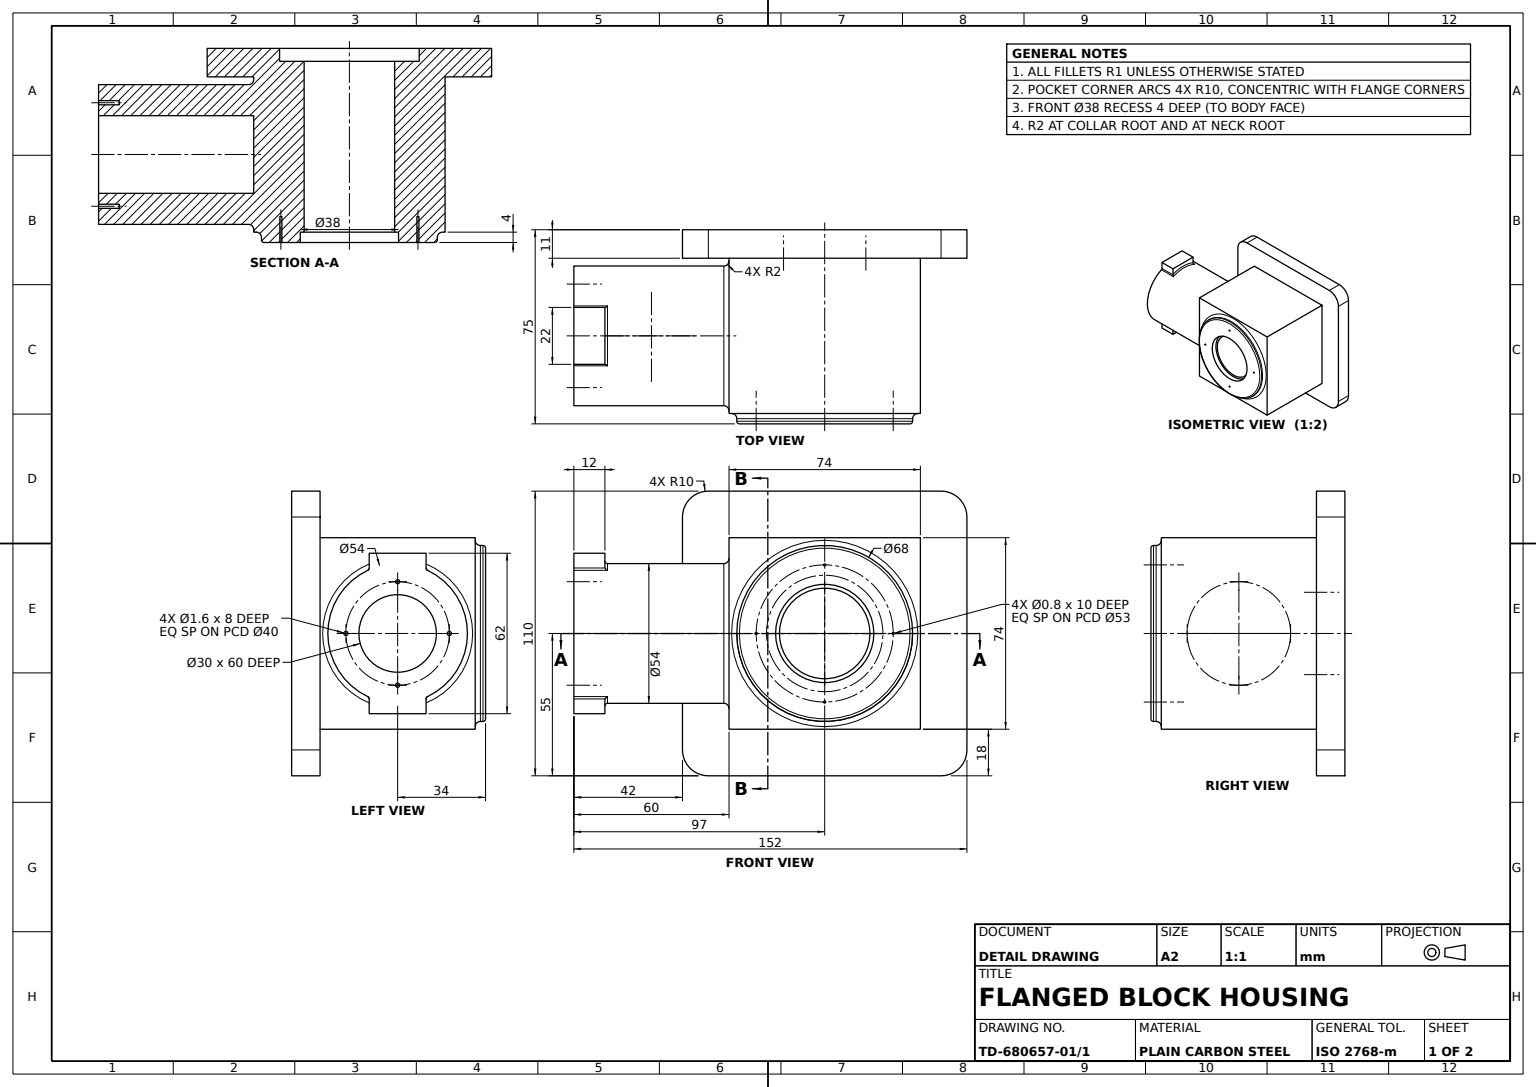
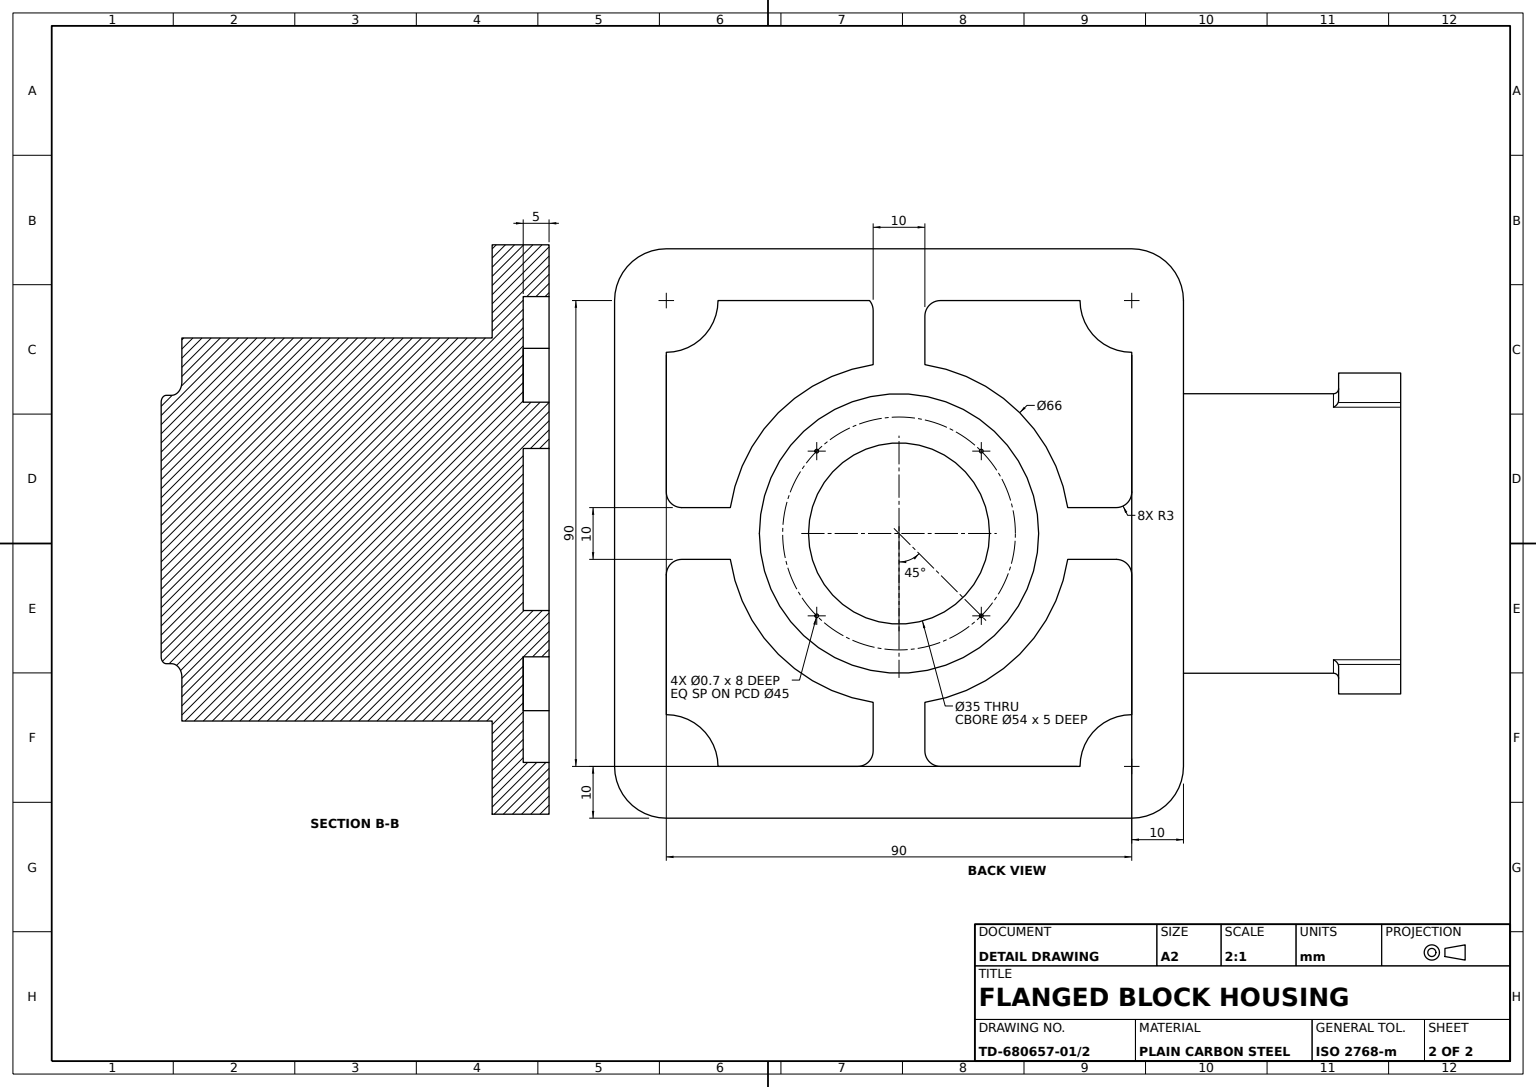
from build123d import *

# Parameters (mm, degrees)
MOUNTING_FLANGE_SKETCH_W      = 110
MOUNTING_FLANGE_SKETCH_H      = 110
MOUNTING_FLANGE_110X110_DEPTH = 11
FLANGE_RECESS_SKETCH_R        = 27
FLANGE_RECESS_SKETCH_R_2      = 17.5
FLANGE_RECESS_DEPTH           = 5
BODY_BLOCK_74X74_DEPTH        = 60
NECK_SKETCH_R                 = 27
CYLINDRICAL_NECK_54_DEPTH     = 60
NECK_START                    = 12
NECK_KEY_LUG_DEPTH            = 12
NECK_BORE_SKETCH_R            = 15.000462615
NECK_BORE_30_DEPTH            = 60
NECK_MARK_SKETCH_R            = 0.8
NECK_MARK_DEPTH               = 8
NECK_MARK_PATTERN_4X_COUNT    = 4
FRONT_COLLAR_SKETCH_R         = 34
FRONT_COLLAR_SKETCH_R_2       = 19
FRONT_COLLAR_RING_68_DEPTH    = 4
FRONT_BORE_SKETCH_R           = 17.5
FRONT_BORE_35_DEPTH           = 172
COLLAR_MARK_SKETCH_R          = 0.4
COLLAR_MARK_DEPTH             = 10
COLLAR_MARK_PATTERN_4X_COUNT  = 4
RECESS_MARK_SKETCH_R          = 0.35
RECESS_MARK_DEPTH             = 8
RECESS_MARK_PATTERN_4X_COUNT  = 4
FLANGE_CORNER_FILLETS_R10_R   = 10
COLLAR_EDGE_FILLET_R1_R       = 1
COLLAR_ROOT_FILLET_R2_R       = 2
NECK_ROOT_FILLET_R2_R         = 2
KEY_LUG_FILLETS_R1_R          = 1


with BuildPart() as part:
    # Mounting Flange Sketch → Mounting Flange 110x110 (new body)
    with BuildSketch(Plane.XY):
        with Locations((55, 55)):
            Rectangle(MOUNTING_FLANGE_SKETCH_W, MOUNTING_FLANGE_SKETCH_H)
    extrude(amount=MOUNTING_FLANGE_110X110_DEPTH)

    # Flange Recess Sketch → Flange Recess (cut)
    # profile 1 of 5: a face of its own
    with BuildSketch(Plane(origin=(0, 0, 0), x_dir=(-1, 0, 0), z_dir=(0, 0, -1))):
        with Locations((-55, 55)):
            Circle(FLANGE_RECESS_SKETCH_R)
        with Locations((-55, 55)):
            Circle(FLANGE_RECESS_SKETCH_R_2, mode=Mode.SUBTRACT)
    # profile 2 of 5: a face of its own
    with BuildSketch(Plane(origin=(0, 0, 0), x_dir=(-1, 0, 0), z_dir=(0, 0, -1))):
        with BuildLine():
            Line((-50, 13), (-50, 22.380987139))
            ThreePointArc((-50, 22.380987139), (-31.665476221, 31.665476221), (-22.380987139, 50))
            Line((-22.380987139, 50), (-13, 50))
            ThreePointArc((-13, 50), (-10.878679656, 49.121320344), (-10, 47))
            Line((-10, 47), (-10, 20))
            ThreePointArc((-10, 20), (-17.071067812, 17.071067812), (-20, 10))
            Line((-20, 10), (-47, 10))
            ThreePointArc((-47, 10), (-49.121320344, 10.878679656), (-50, 13))
        make_face()
    # profile 3 of 5: a face of its own
    with BuildSketch(Plane(origin=(0, 0, 0), x_dir=(-1, 0, 0), z_dir=(0, 0, -1))):
        with BuildLine():
            Line((-60, 13), (-60, 22.380987139))
            ThreePointArc((-60, 22.380987139), (-78.334523779, 31.665476221), (-87.619012861, 50))
            Line((-87.619012861, 50), (-97, 50))
            ThreePointArc((-97, 50), (-99.121320344, 49.121320344), (-100, 47))
            Line((-100, 47), (-100, 20))
            ThreePointArc((-100, 20), (-92.928932188, 17.071067812), (-90, 10))
            Line((-90, 10), (-63, 10))
            ThreePointArc((-63, 10), (-60.878679656, 10.878679656), (-60, 13))
        make_face()
    # profile 4 of 5: a face of its own
    with BuildSketch(Plane(origin=(0, 0, 0), x_dir=(-1, 0, 0), z_dir=(0, 0, -1))):
        with BuildLine():
            Line((-97, 60), (-87.619012861, 60))
            ThreePointArc((-87.619012861, 60), (-78.334523779, 78.334523779), (-60, 87.619012861))
            Line((-60, 87.619012861), (-60, 98.076241066))
            ThreePointArc((-60, 98.076241066), (-60.179896648, 99.099479593), (-60.698011389, 100))
            Line((-60.698011389, 100), (-90, 100))
            ThreePointArc((-90, 100), (-92.928932188, 92.928932188), (-100, 90))
            Line((-100, 90), (-100, 63))
            ThreePointArc((-100, 63), (-99.121320344, 60.878679656), (-97, 60))
        make_face()
    # profile 5 of 5: a face of its own
    with BuildSketch(Plane(origin=(0, 0, 0), x_dir=(-1, 0, 0), z_dir=(0, 0, -1))):
        with BuildLine():
            Line((-50, 97), (-50, 87.619012861))
            ThreePointArc((-50, 87.619012861), (-31.665476221, 78.334523779), (-22.380987139, 60))
            Line((-22.380987139, 60), (-13, 60))
            ThreePointArc((-13, 60), (-10.878679656, 60.878679656), (-10, 63))
            Line((-10, 63), (-10, 90))
            ThreePointArc((-10, 90), (-17.071067812, 92.928932188), (-20, 100))
            Line((-20, 100), (-47, 100))
            ThreePointArc((-47, 100), (-49.121320344, 99.121320344), (-50, 97))
        make_face()
    extrude(amount=-FLANGE_RECESS_DEPTH, mode=Mode.SUBTRACT)

    # Body Block Sketch → Body Block 74x74 (add)
    with BuildSketch(Plane.XY.offset(11)):
        Polygon((55, 18), (92, 18), (92, 92), (18, 92), (18, 18), align=None)
    extrude(amount=BODY_BLOCK_74X74_DEPTH)

    # Neck Sketch → Cylindrical Neck Ø54 (add)
    with BuildSketch(Plane.ZY.offset(-18)):
        with Locations(Location((41, 55, 0), (0, 0, 180))):
            Circle(NECK_SKETCH_R)
    extrude(amount=CYLINDRICAL_NECK_54_DEPTH)

    # Key Lug Sketch → Neck Key Lug (add)
    with BuildSketch(Plane(origin=(-42, 0, 0), x_dir=(0, 0, -1), z_dir=(1, 0, 0)).offset(NECK_START)):
        with BuildLine():
            Line((-41, 86), (-30, 86))
            Line((-30, 86), (-30, 79.657656012))
            ThreePointArc((-30, 79.657656012), (-41, 82), (-52, 79.657656012))
            Line((-52, 79.657656012), (-52, 86))
            Line((-52, 86), (-41, 86))
        make_face()
    neck_key_lug = extrude(amount=-NECK_KEY_LUG_DEPTH)

    # Key Lug Mirror: Neck Key Lug across plane
    add(neck_key_lug.mirror(Plane.ZX.offset(55)))

    # Neck Bore Sketch → Neck Bore Ø30 (cut)
    with BuildSketch(Plane.ZY.offset(42)):
        with Locations((41, 55)):
            Circle(NECK_BORE_SKETCH_R)
    extrude(amount=-NECK_BORE_30_DEPTH, mode=Mode.SUBTRACT)

    # Neck Mark Sketch → Neck Mark (cut)
    with BuildSketch(Plane.ZY.offset(42)):
        with Locations((61, 55)):
            Circle(NECK_MARK_SKETCH_R)
    neck_mark = extrude(amount=-NECK_MARK_DEPTH, mode=Mode.SUBTRACT)

    # Neck Mark Pattern 4x: Neck Mark ×4 about axis
    neck_mark_pattern_4x_axis = Axis((0, 55, 41), (1, 0, 0))
    for i in range(1, NECK_MARK_PATTERN_4X_COUNT):
        add(neck_mark.rotate(neck_mark_pattern_4x_axis, i * 360 / NECK_MARK_PATTERN_4X_COUNT), mode=Mode.SUBTRACT)

    # Front Collar Sketch → Front Collar Ring Ø68 (add)
    with BuildSketch(Plane.XY.offset(71)):
        with Locations((55, 55)):
            Circle(FRONT_COLLAR_SKETCH_R)
        with Locations((55, 55)):
            Circle(FRONT_COLLAR_SKETCH_R_2, mode=Mode.SUBTRACT)
    extrude(amount=FRONT_COLLAR_RING_68_DEPTH)

    # Front Bore Sketch → Front Bore Ø35 (cut, through all)
    with BuildSketch(Plane.XY.offset(71)):
        with Locations((55, 55)):
            Circle(FRONT_BORE_SKETCH_R)
    extrude(amount=-FRONT_BORE_35_DEPTH, mode=Mode.SUBTRACT)

    # Collar Mark Sketch → Collar Mark (cut)
    with BuildSketch(Plane.XY.offset(75)):
        with Locations((55, 81.5)):
            Circle(COLLAR_MARK_SKETCH_R)
    collar_mark = extrude(amount=-COLLAR_MARK_DEPTH, mode=Mode.SUBTRACT)

    # Collar Mark Pattern 4x: Collar Mark ×4 about axis
    collar_mark_pattern_4x_axis = Axis((55, 55, 0), (0, 0, 1))
    for i in range(1, COLLAR_MARK_PATTERN_4X_COUNT):
        add(collar_mark.rotate(collar_mark_pattern_4x_axis, i * 360 / COLLAR_MARK_PATTERN_4X_COUNT), mode=Mode.SUBTRACT)

    # Recess Mark Sketch → Recess Mark (cut)
    with BuildSketch(Plane(origin=(0, 0, 5), x_dir=(-1, 0, 0), z_dir=(0, 0, -1))):
        with Locations((-70.909902577, 70.909902577)):
            Circle(RECESS_MARK_SKETCH_R)
    recess_mark = extrude(amount=-RECESS_MARK_DEPTH, mode=Mode.SUBTRACT)

    # Recess Mark Pattern 4x: Recess Mark ×4 about axis
    recess_mark_pattern_4x_axis = Axis((55, 55, 0), (0, 0, 1))
    for i in range(1, RECESS_MARK_PATTERN_4X_COUNT):
        add(recess_mark.rotate(recess_mark_pattern_4x_axis, i * 360 / RECESS_MARK_PATTERN_4X_COUNT), mode=Mode.SUBTRACT)

    # Flange Corner Fillets R10
    flange_corner_fillets_r10_edges = [part.edges().sort_by_distance(p)[0] for p in [
        (0, 110, 5.5),
        (110, 110, 5.5),
        (110, 0, 5.5),
        (0, 0, 5.5),
    ]]
    fillet(flange_corner_fillets_r10_edges, radius=FLANGE_CORNER_FILLETS_R10_R)

    # Collar Edge Fillet R1
    collar_edge_fillet_r1_edges = [part.edges().sort_by_distance(p)[0] for p in [
        (21, 55, 75),
    ]]
    fillet(collar_edge_fillet_r1_edges, radius=COLLAR_EDGE_FILLET_R1_R)

    # Collar Root Fillet R2
    collar_root_fillet_r2_edges = [part.edges().sort_by_distance(p)[0] for p in [
        (21, 55, 71),
    ]]
    fillet(collar_root_fillet_r2_edges, radius=COLLAR_ROOT_FILLET_R2_R)

    # Neck Root Fillet R2
    neck_root_fillet_r2_edges = [part.edges().sort_by_distance(p)[0] for p in [
        (18, 55, 68),
    ]]
    fillet(neck_root_fillet_r2_edges, radius=NECK_ROOT_FILLET_R2_R)

    # Key Lug Fillets R1
    key_lug_fillets_r1_edges = [part.edges().sort_by_distance(p)[0] for p in [
        (-36, 79.657656012, 52),
        (-36, 79.657656012, 30),
        (-30, 82, 41),
        (-30, 28, 41),
        (-36, 30.342343988, 30),
        (-36, 30.342343988, 52),
    ]]
    fillet(key_lug_fillets_r1_edges, radius=KEY_LUG_FILLETS_R1_R)


solid = part.part
